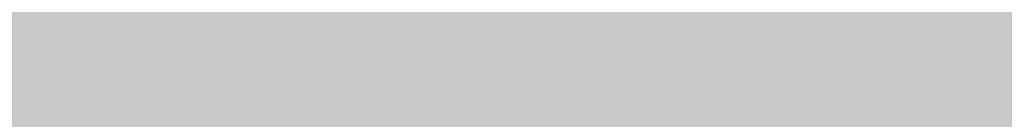
# Model space of a CAD drawing. Units: millimetres. Extents: x 0 to 2267, y 0 to 1823.
# Tile 104 of 256: x 1600.369 to 1605.705, y 1231.521 to 1232.061. Entities that reach past the tile are written whole.
import ezdxf

# ---------------------------------------------------------------- set-up
doc = ezdxf.new("R2010")
doc.units = ezdxf.units.MM
doc.header["$MEASUREMENT"] = 0
doc.layers.add('M-DIMS', color=2, linetype='Continuous', lineweight=25)
doc.layers.add('M-HATC', color=252, linetype='Continuous', lineweight=18)
doc.styles.get("Standard").update_dxf_attribs({"font": 'arial.ttf'})
doc.dimstyles.get("Standard").update_dxf_attribs({"dimtxt": 7, "dimasz": 4, "dimexe": 0.18, "dimexo": 0.0625, "dimgap": 0.09, "dimtad": 0, "dimdec": 0, "dimzin": 0, "dimdsep": 46, "dimtxsty": 'Standard', "dimcen": 0.09, "dimadec": 0, "dimazin": 0, "dimtfac": 1, "dimtdec": 0, "dimtofl": 0, "dimtmove": 0, "dimatfit": 3, "dimfxl": 1, "dimtolj": 1, "dimtzin": 0, "dimarcsym": 0})

# ---------------------------------------------------------------- blocks, each defined once
blk = doc.blocks.new('*D19')
at = {"layer": 'Defpoints', "color": 0, "transparency": 16777216}
for p in [(1605.3399, 1483.3044), (1445.5291, 1333.8851)]:
    blk.add_point(p, dxfattribs=at)
at = {"layer": 'M-DIMS', "color": 0, "lineweight": -2, "transparency": 16777216}
for p, q in [((1605.3399, 1483.2144), (1605.3399, 1483.3944)), ((1605.2499, 1483.3044), (1605.4299, 1483.3044)), ((1366.3244, 1259.8306), (1442.6072, 1331.1532))]:
    blk.add_line(p, q, dxfattribs=at)
at = {"layer": 'M-DIMS', "color": 0, "transparency": 16777216}
blk.add_solid([(1442.1519, 1331.6402), (1443.0625, 1330.6663), (1445.5291, 1333.8851)], dxfattribs=at)
at = {"layer": 'M-DIMS', "color": 0, "transparency": 16777216, "insert": (1349.6425, 1244.2335), "char_height": 7, "attachment_point": 5, "rotation": 43.0753}
blk.add_mtext('\\A1;2X R218.8', dxfattribs=at)

msp = doc.modelspace()

# ---------------------------------------------------------------- hatches: boundary and pattern name
at = {"layer": 'M-HATC'}
h = msp.add_hatch(color=256, dxfattribs=at)
h.dxf.hatch_style = 1
h.paths.add_polyline_path([(2055.771, 1603.062), (1381.0868, 1603.062), (1381.0868, 1598.062), (2055.771, 1598.062)])
h.paths.add_polyline_path([(2055.771, 1598.062), (1381.0868, 1598.062), (1381.0868, 1593.062), (2055.771, 1593.062)])
h.paths.add_polyline_path([(2051.3074, 1536.7609), (1385.5504, 1536.7609), (1385.5504, 1526.7609), (1387.5504, 1526.7609), (1388.5366, 1525.0528), (1385.3319, 1521.2335), (1385.3319, 1521.2226), (2050.2542, 1522.7491), (2048.3212, 1525.0528), (2049.3074, 1526.7609), (2051.3074, 1526.7609)])
edge = h.paths.add_edge_path()
edge.add_arc((1847.5345, 1379.1492), 135, 222.603061, 222.890851, ccw=False)
edge.add_line((1748.1663, 1287.7656), (1683.0921, 1287.7656))
edge.add_arc((1583.7239, 1379.1492), 135, 317.109149, 317.396939, ccw=False)
edge.add_arc((1678.9686, 1290.6707), 5, 222.8909, 317.1091, ccw=False)
edge.add_arc((1774.2133, 1379.1492), 135, 222.603061, 222.890851, ccw=False)
edge.add_line((1674.8451, 1287.7656), (1609.7709, 1287.7656))
edge.add_arc((1510.4027, 1379.1492), 135, 317.109149, 317.396939, ccw=False)
edge.add_arc((1605.6474, 1290.6707), 5, 222.8909, 317.1091, ccw=False)
edge.add_arc((1700.8921, 1379.1492), 135, 222.603061, 222.890851, ccw=False)
edge.add_line((1601.5239, 1287.7656), (1536.4497, 1287.7656))
edge.add_arc((1437.0815, 1379.1492), 135, 317.109149, 317.396939, ccw=False)
edge.add_arc((1532.3262, 1290.6707), 5, 222.8909, 317.1091, ccw=False)
edge.add_arc((1627.5709, 1379.1492), 135, 222.603061, 222.890851, ccw=False)
edge.add_line((1528.2027, 1287.7656), (1505.9289, 1287.7656))
edge.add_spline(control_points=[(1505.9289, 1287.7656), (1504.2622, 1287.7656), (1504.2622, 1282.7656), (1505.9289, 1282.7656)], knot_values=[0, 0, 0, 0, 5, 5, 5, 5], degree=3, periodic=0)
edge.add_line((1505.9289, 1282.7656), (1930.9289, 1282.7656))
edge.add_spline(control_points=[(1930.9289, 1282.7656), (1932.5956, 1282.7656), (1932.5956, 1287.7656), (1930.9289, 1287.7656)], knot_values=[0, 0, 0, 0, 5, 5, 5, 5], degree=3, periodic=0)
edge.add_line((1930.9289, 1287.7656), (1903.0557, 1287.7656))
edge.add_arc((1803.6875, 1379.1492), 135, 317.109149, 317.396939, ccw=False)
edge.add_arc((1898.9322, 1290.6707), 5, 222.8909, 317.1091, ccw=False)
edge.add_arc((1994.1769, 1379.1492), 135, 222.603061, 222.890851, ccw=False)
edge.add_line((1894.8087, 1287.7656), (1829.7345, 1287.7656))
edge.add_arc((1730.3663, 1379.1492), 135, 317.109149, 317.396939, ccw=False)
edge.add_arc((1825.611, 1290.6707), 5, 222.8909, 317.1091, ccw=False)
edge.add_arc((1920.8557, 1379.1492), 135, 222.603061, 222.890851, ccw=False)
edge.add_line((1821.4875, 1287.7656), (1756.4133, 1287.7656))
edge.add_arc((1657.0451, 1379.1492), 135, 317.109149, 317.396939, ccw=False)
edge.add_arc((1752.2898, 1290.6707), 5, 222.8909, 317.1091, ccw=False)
edge = h.paths.add_edge_path()
edge.add_spline(control_points=[(1843.4289, 1227.2475), (1845.0956, 1227.2475), (1845.0956, 1232.2475), (1843.4289, 1232.2475)], knot_values=[0, 0, 0, 0, 5, 5, 5, 5], degree=3, periodic=0)
edge.add_line((1843.4289, 1232.2475), (1593.4289, 1232.2475))
edge.add_spline(control_points=[(1593.4289, 1232.2475), (1591.7622, 1232.2475), (1591.7622, 1227.2475), (1593.4289, 1227.2475)], knot_values=[0, 0, 0, 0, 5, 5, 5, 5], degree=3, periodic=0)
edge.add_line((1593.4289, 1227.2475), (1843.4289, 1227.2475))
h.paths.add_polyline_path([(1905.9289, 1127.4171), (1530.9289, 1127.4171, 0.414214), (1520.9289, 1117.4171), (1530.9289, 1117.4171), (1915.9289, 1117.4171, 0.414214)])
edge = h.paths.add_edge_path()
edge.add_arc((1397.0858, 1498.4078), 12.7299, 90.78215, 190.87871, ccw=False)
edge.add_line((1396.912, 1511.1365), (1428.0097, 1511.3488))
edge.add_line((1428.0097, 1511.3488), (1433.0097, 1511.3488))
edge.add_line((1433.0097, 1511.3488), (1434.439, 1511.3488))
edge.add_arc((1419.474, 1498.0804), 20, 41.561, 74.08211)
edge.add_line((1424.9592, 1517.3135), (1399.9351, 1517.2561))
edge.add_spline(control_points=[(1399.9307, 1517.2561), (1399.884, 1517.2131), (1399.8328, 1517.1689), (1399.7774, 1517.1236)], knot_values=[11.567499, 11.567499, 11.567499, 11.567499, 11.814249, 11.814249, 11.814249, 11.814249], degree=3, periodic=0)
edge.add_spline(control_points=[(1399.6328, 1517.0099), (1399.5831, 1516.9721), (1399.5307, 1516.9338), (1399.4759, 1516.8947)], knot_values=[11.167718, 11.167718, 11.167718, 11.167718, 11.365188, 11.365188, 11.365188, 11.365188], degree=3, periodic=0)
edge.add_spline(control_points=[(1399.3398, 1516.8001), (1399.1514, 1516.6719), (1398.9384, 1516.5377), (1398.704, 1516.3994)], knot_values=[10.376405, 10.376405, 10.376405, 10.376405, 11.00994, 11.00994, 11.00994, 11.00994], degree=3, periodic=0)
edge.add_spline(control_points=[(1398.6572, 1516.3719), (1398.5789, 1516.326), (1398.4983, 1516.2797), (1398.4155, 1516.2331)], knot_values=[10.125175, 10.125175, 10.125175, 10.125175, 10.334406, 10.334406, 10.334406, 10.334406], degree=3, periodic=0)
edge.add_spline(control_points=[(1398.2642, 1516.1487), (1398.196, 1516.1111), (1398.1263, 1516.0732), (1398.0555, 1516.0351)], knot_values=[9.832246, 9.832246, 9.832246, 9.832246, 9.999658, 9.999658, 9.999658, 9.999658], degree=3, periodic=0)
edge.add_spline(control_points=[(1397.9987, 1516.0048), (1397.7312, 1515.8621), (1397.446, 1515.7171), (1397.1466, 1515.5714)], knot_values=[9.161808, 9.161808, 9.161808, 9.161808, 9.787769, 9.787769, 9.787769, 9.787769], degree=3, periodic=0)
edge.add_spline(control_points=[(1397.1466, 1515.5714), (1396.8418, 1515.423), (1396.5222, 1515.274), (1396.1914, 1515.1262)], knot_values=[8.524455, 8.524455, 8.524455, 8.524455, 9.161808, 9.161808, 9.161808, 9.161808], degree=3, periodic=0)
edge.add_spline(control_points=[(1396.0777, 1515.0756), (1395.9854, 1515.0348), (1395.8922, 1514.994), (1395.7983, 1514.9534)], knot_values=[8.275193, 8.275193, 8.275193, 8.275193, 8.451726, 8.451726, 8.451726, 8.451726], degree=3, periodic=0)
edge.add_spline(control_points=[(1395.6018, 1514.8691), (1395.4997, 1514.8257), (1395.3968, 1514.7824), (1395.2932, 1514.7394)], knot_values=[7.962917, 7.962917, 7.962917, 7.962917, 8.152764, 8.152764, 8.152764, 8.152764], degree=3, periodic=0)
edge.add_spline(control_points=[(1395.2116, 1514.7057), (1394.8278, 1514.5475), (1394.4345, 1514.3929), (1394.0364, 1514.2442)], knot_values=[7.21254, 7.21254, 7.21254, 7.21254, 7.913148, 7.913148, 7.913148, 7.913148], degree=3, periodic=0)
edge.add_spline(control_points=[(1394.0364, 1514.2442), (1393.7076, 1514.1214), (1393.3754, 1514.0027), (1393.0427, 1513.8895)], knot_values=[6.633733, 6.633733, 6.633733, 6.633733, 7.21254, 7.21254, 7.21254, 7.21254], degree=3, periodic=0)
edge.add_spline(control_points=[(1392.8214, 1513.815), (1392.7198, 1513.7812), (1392.6181, 1513.7479), (1392.5166, 1513.7152)], knot_values=[6.328796, 6.328796, 6.328796, 6.328796, 6.505493, 6.505493, 6.505493, 6.505493], degree=3, periodic=0)
edge.add_spline(control_points=[(1392.5166, 1513.7152), (1392.3187, 1513.6515), (1392.1212, 1513.59), (1391.9244, 1513.531)], knot_values=[5.984605, 5.984605, 5.984605, 5.984605, 6.328796, 6.328796, 6.328796, 6.328796], degree=3, periodic=0)
edge.add_spline(control_points=[(1391.7915, 1513.4915), (1391.3122, 1513.3501), (1390.8384, 1513.2239), (1390.3784, 1513.1171)], knot_values=[5.066697, 5.066697, 5.066697, 5.066697, 5.907055, 5.907055, 5.907055, 5.907055], degree=3, periodic=0)
edge.add_spline(control_points=[(1390.3784, 1513.1171), (1390.1797, 1513.071), (1389.9836, 1513.0284), (1389.7907, 1512.9899)], knot_values=[4.70367, 4.70367, 4.70367, 4.70367, 5.066695, 5.066695, 5.066695, 5.066695], degree=3, periodic=0)
edge.add_spline(control_points=[(1389.422, 1512.9204), (1389.2459, 1512.8892), (1389.0729, 1512.8617), (1388.9036, 1512.8381)], knot_values=[4.130571, 4.130571, 4.130571, 4.130571, 4.469816, 4.469816, 4.469816, 4.469816], degree=3, periodic=0)
edge.add_spline(control_points=[(1388.9036, 1512.8381), (1388.591, 1512.7946), (1388.2911, 1512.7644), (1388.0071, 1512.7494)], knot_values=[3.504031, 3.504031, 3.504031, 3.504031, 4.130571, 4.130571, 4.130571, 4.130571], degree=3, periodic=0)
edge.add_spline(control_points=[(1387.9356, 1512.7459), (1387.8538, 1512.7423), (1387.7733, 1512.74), (1387.6944, 1512.739)], knot_values=[3.268866, 3.268866, 3.268866, 3.268866, 3.451164, 3.451164, 3.451164, 3.451164], degree=3, periodic=0)
edge.add_spline(control_points=[(1387.3351, 1512.7443), (1387.2076, 1512.7499), (1387.0847, 1512.7597), (1386.967, 1512.7739)], knot_values=[2.670686, 2.670686, 2.670686, 2.670686, 2.984, 2.984, 2.984, 2.984], degree=3, periodic=0)
edge.add_spline(control_points=[(1386.8327, 1512.7922), (1386.8209, 1512.7941), (1386.8092, 1512.7959), (1386.7975, 1512.7979)], knot_values=[2.516981, 2.516981, 2.516981, 2.516981, 2.549528, 2.549528, 2.549528, 2.549528], degree=3, periodic=0)
edge.add_spline(control_points=[(1386.4526, 1512.8735), (1386.4257, 1512.881), (1386.3993, 1512.889), (1386.3733, 1512.8972)], knot_values=[2.095869, 2.095869, 2.095869, 2.095869, 2.17941, 2.17941, 2.17941, 2.17941], degree=3, periodic=0)
edge.add_spline(control_points=[(1386.0691, 1513.0189), (1386.0634, 1513.0217), (1386.0577, 1513.0246), (1386.052, 1513.0275)], knot_values=[1.72453, 1.72453, 1.72453, 1.72453, 1.745933, 1.745933, 1.745933, 1.745933], degree=3, periodic=0)
edge.add_arc((1399.474, 1498.0804), 20, 131.82432, 180)
edge.add_arc((1630.3336, 1505.5484), 250.9708, 181.705176, 236.427975)
edge.add_arc((1605.3399, 1483.3044), 218.7822, 238.660829, 243.34961)
edge.add_arc((1647.0911, 1510.3592), 262.8986, 183.129836, 237.853442, ccw=False)
h.paths.add_polyline_path([(1406.5369, 1391.9644, 0.149382), (1491.5506, 1296.4418, -0.129517)], flags=17)
edge = h.paths.add_edge_path()
edge.add_arc((2037.3838, 1498.0804), 20, 0, 48.26587)
edge.add_spline(control_points=[(2050.6973, 1513.0052), (2050.6512, 1512.9847), (2050.6034, 1512.9655), (2050.5539, 1512.9477)], knot_values=[1.835652, 1.835652, 1.835652, 1.835652, 2.000781, 2.000781, 2.000781, 2.000781], degree=3, periodic=0)
edge.add_spline(control_points=[(2050.4616, 1512.9166), (2050.479, 1512.9221), (2050.4963, 1512.9277), (2050.5133, 1512.9335)], knot_values=[2.045477, 2.045477, 2.045477, 2.045477, 2.101389, 2.101389, 2.101389, 2.101389], degree=3, periodic=0)
edge.add_spline(control_points=[(2050.129, 1512.8342), (2050.1984, 1512.8473), (2050.2657, 1512.8623), (2050.3308, 1512.8792)], knot_values=[2.237629, 2.237629, 2.237629, 2.237629, 2.435841, 2.435841, 2.435841, 2.435841], degree=3, periodic=0)
edge.add_spline(control_points=[(2050.0946, 1512.8278), (2050.1061, 1512.8299), (2050.1176, 1512.832), (2050.129, 1512.8342)], knot_values=[2.435841, 2.435841, 2.435841, 2.435841, 2.468321, 2.468321, 2.468321, 2.468321], degree=3, periodic=0)
edge.add_spline(control_points=[(2049.7843, 1512.7851), (2049.8552, 1512.7922), (2049.9243, 1512.8008), (2049.9917, 1512.8109)], knot_values=[2.563852, 2.563852, 2.563852, 2.563852, 2.748541, 2.748541, 2.748541, 2.748541], degree=3, periodic=0)
edge.add_spline(control_points=[(2049.4052, 1512.7617), (2049.5364, 1512.7653), (2049.6629, 1512.773), (2049.7843, 1512.7851)], knot_values=[2.748541, 2.748541, 2.748541, 2.748541, 3.064882, 3.064882, 3.064882, 3.064882], degree=3, periodic=0)
edge.add_spline(control_points=[(2049.1698, 1512.7597), (2049.2336, 1512.7591), (2049.2965, 1512.7594), (2049.3584, 1512.7606)], knot_values=[3.102309, 3.102309, 3.102309, 3.102309, 3.2503, 3.2503, 3.2503, 3.2503], degree=3, periodic=0)
edge.add_spline(control_points=[(2048.8573, 1512.7691), (2048.9638, 1512.7638), (2049.068, 1512.7606), (2049.1698, 1512.7597)], knot_values=[3.2503, 3.2503, 3.2503, 3.2503, 3.486069, 3.486069, 3.486069, 3.486069], degree=3, periodic=0)
edge.add_spline(control_points=[(2048.6924, 1512.7789), (2048.3729, 1512.8009), (2048.0345, 1512.8411), (2047.6817, 1512.897)], knot_values=[3.606429, 3.606429, 3.606429, 3.606429, 4.2989, 4.2989, 4.2989, 4.2989], degree=3, periodic=0)
edge.add_spline(control_points=[(2047.6817, 1512.897), (2047.5458, 1512.9185), (2047.4077, 1512.9424), (2047.2678, 1512.9685)], knot_values=[4.2989, 4.2989, 4.2989, 4.2989, 4.565769, 4.565769, 4.565769, 4.565769], degree=3, periodic=0)
edge.add_spline(control_points=[(2047.2678, 1512.9685), (2047.1449, 1512.9914), (2047.0207, 1513.016), (2046.8951, 1513.0422)], knot_values=[4.565769, 4.565769, 4.565769, 4.565769, 4.799971, 4.799971, 4.799971, 4.799971], degree=3, periodic=0)
edge.add_spline(control_points=[(2046.8951, 1513.0422), (2046.5286, 1513.1188), (2046.1513, 1513.209), (2045.7676, 1513.3107)], knot_values=[4.799971, 4.799971, 4.799971, 4.799971, 5.483718, 5.483718, 5.483718, 5.483718], degree=3, periodic=0)
edge.add_spline(control_points=[(2045.7676, 1513.3107), (2045.3724, 1513.4154), (2044.9704, 1513.5322), (2044.5662, 1513.6588)], knot_values=[5.483718, 5.483718, 5.483718, 5.483718, 6.187866, 6.187866, 6.187866, 6.187866], degree=3, periodic=0)
edge.add_spline(control_points=[(2044.5662, 1513.6588), (2044.4149, 1513.7061), (2044.2633, 1513.7549), (2044.1116, 1513.8048)], knot_values=[6.187866, 6.187866, 6.187866, 6.187866, 6.451551, 6.451551, 6.451551, 6.451551], degree=3, periodic=0)
edge.add_spline(control_points=[(2044.1116, 1513.8048), (2043.9967, 1513.8427), (2043.8817, 1513.8813), (2043.7668, 1513.9205)], knot_values=[6.451551, 6.451551, 6.451551, 6.451551, 6.651434, 6.651434, 6.651434, 6.651434], degree=3, periodic=0)
edge.add_spline(control_points=[(2043.7668, 1513.9205), (2043.3716, 1514.0554), (2042.9774, 1514.1979), (2042.5886, 1514.3458)], knot_values=[6.651434, 6.651434, 6.651434, 6.651434, 7.338879, 7.338879, 7.338879, 7.338879], degree=3, periodic=0)
edge.add_spline(control_points=[(2042.5886, 1514.3458), (2042.1643, 1514.5071), (2041.7465, 1514.6749), (2041.3409, 1514.846)], knot_values=[7.338879, 7.338879, 7.338879, 7.338879, 8.089209, 8.089209, 8.089209, 8.089209], degree=3, periodic=0)
edge.add_spline(control_points=[(2041.3409, 1514.846), (2041.1028, 1514.9465), (2040.869, 1515.0481), (2040.6405, 1515.1502)], knot_values=[8.089209, 8.089209, 8.089209, 8.089209, 8.529587, 8.529587, 8.529587, 8.529587], degree=3, periodic=0)
edge.add_spline(control_points=[(2040.51, 1515.2089), (2040.0824, 1515.4022), (2039.6747, 1515.5971), (2039.295, 1515.7894)], knot_values=[8.613818, 8.613818, 8.613818, 8.613818, 9.44571, 9.44571, 9.44571, 9.44571], degree=3, periodic=0)
edge.add_spline(control_points=[(2039.295, 1515.7894), (2039.0618, 1515.9075), (2038.8391, 1516.0246), (2038.6288, 1516.1398)], knot_values=[9.44571, 9.44571, 9.44571, 9.44571, 9.956404, 9.956404, 9.956404, 9.956404], degree=3, periodic=0)
edge.add_spline(control_points=[(2038.6288, 1516.1398), (2038.5187, 1516.2001), (2038.4121, 1516.2598), (2038.309, 1516.3189)], knot_values=[9.956404, 9.956404, 9.956404, 9.956404, 10.223542, 10.223542, 10.223542, 10.223542], degree=3, periodic=0)
edge.add_spline(control_points=[(2038.309, 1516.3189), (2038.2138, 1516.3735), (2038.1216, 1516.4276), (2038.0328, 1516.481)], knot_values=[10.223542, 10.223542, 10.223542, 10.223542, 10.47051, 10.47051, 10.47051, 10.47051], degree=3, periodic=0)
edge.add_spline(control_points=[(2038.0328, 1516.481), (2037.7855, 1516.6296), (2037.5639, 1516.773), (2037.3722, 1516.909)], knot_values=[10.47051, 10.47051, 10.47051, 10.47051, 11.15767, 11.15767, 11.15767, 11.15767], degree=3, periodic=0)
edge.add_spline(control_points=[(2037.3722, 1516.909), (2037.2789, 1516.9752), (2037.1927, 1517.0396), (2037.1142, 1517.102)], knot_values=[11.15767, 11.15767, 11.15767, 11.15767, 11.49227, 11.49227, 11.49227, 11.49227], degree=3, periodic=0)
edge.add_spline(control_points=[(2036.8564, 1517.3259), (2036.9148, 1517.2692), (2036.9814, 1517.2103), (2037.0557, 1517.1492)], knot_values=[11.577341, 11.577341, 11.577341, 11.577341, 11.91035, 11.91035, 11.91035, 11.91035], degree=3, periodic=0)
edge.add_spline(control_points=[(2036.8074, 1517.3748), (2036.823, 1517.3587), (2036.8393, 1517.3424), (2036.8564, 1517.3259)], knot_values=[11.91035, 11.91035, 11.91035, 11.91035, 12.007402, 12.007402, 12.007402, 12.007402], degree=3, periodic=0)
edge.add_spline(control_points=[(2036.7017, 1517.494), (2036.7104, 1517.483), (2036.7196, 1517.4719), (2036.7291, 1517.4606)], knot_values=[12.184155, 12.184155, 12.184155, 12.184155, 12.255409, 12.255409, 12.255409, 12.255409], degree=3, periodic=0)
edge.add_spline(control_points=[(2036.6159, 1517.6205), (2036.62, 1517.613), (2036.6243, 1517.6055), (2036.6289, 1517.5979)], knot_values=[12.487913, 12.487913, 12.487913, 12.487913, 12.541035, 12.541035, 12.541035, 12.541035], degree=3, periodic=0)
edge.add_spline(control_points=[(2036.5635, 1517.786), (2036.5637, 1517.7794), (2036.5642, 1517.7726), (2036.565, 1517.7658)], knot_values=[12.911761, 12.911761, 12.911761, 12.911761, 12.968286, 12.968286, 12.968286, 12.968286], degree=3, periodic=0)
edge.add_spline(control_points=[(2036.6166, 1517.9304), (2036.6125, 1517.9259), (2036.6086, 1517.9212), (2036.6049, 1517.9165)], knot_values=[13.382527, 13.382527, 13.382527, 13.382527, 13.433791, 13.433791, 13.433791, 13.433791], degree=3, periodic=0)
edge.add_spline(control_points=[(2036.749, 1518.017), (2036.7361, 1518.0116), (2036.7239, 1518.006), (2036.7124, 1518.0002)], knot_values=[13.726299, 13.726299, 13.726299, 13.726299, 13.809928, 13.809928, 13.809928, 13.809928], degree=3, periodic=0)
edge.add_spline(control_points=[(2036.8604, 1518.0528), (2036.8386, 1518.0474), (2036.8181, 1518.0416), (2036.7988, 1518.0353)], knot_values=[13.910887, 13.910887, 13.910887, 13.910887, 14.02153, 14.02153, 14.02153, 14.02153], degree=3, periodic=0)
edge.add_line((2036.9639, 1518.0804), (2032.3838, 1518.0804))
edge.add_line((2032.3838, 1518.0804), (2027.3838, 1518.0804))
edge.add_line((2027.3838, 1518.0804), (2022.3838, 1518.0804))
edge.add_line((2022.3838, 1518.0804), (2017.3838, 1518.0804))
edge.add_arc((2017.3838, 1498.0804), 20, 90, 138.439)
edge.add_line((2002.4188, 1511.3488), (2003.8481, 1511.3488))
edge.add_line((2003.8481, 1511.3488), (2008.8481, 1511.3488))
edge.add_line((2008.8481, 1511.3488), (2039.772, 1511.1377))
edge.add_arc((2039.772, 1498.4078), 12.7299, -10.87871, 90, ccw=False)
edge.add_arc((1789.7668, 1510.3592), 262.8986, 302.146558, 356.870164, ccw=False)
edge.add_arc((1831.5179, 1483.3044), 218.7822, 296.65039, 301.339171)
edge.add_arc((1806.5242, 1505.5484), 250.9708, 303.572025, 358.294824)
h.paths.add_polyline_path([(2030.321, 1391.9644, -0.129517), (1945.3072, 1296.4418, 0.149382)], flags=17)
edge = h.paths.add_edge_path()
edge.add_spline(control_points=[(2037.2464, 1518.0821), (2037.2898, 1518.081), (2037.3355, 1518.0804), (2037.3838, 1518.0804)], knot_values=[0.000012, 0.000012, 0.000012, 0.000012, 0.144754, 0.144754, 0.144754, 0.144754], degree=3, periodic=0)
edge.add_line((2037.3357, 1518.0804), (2037.0096, 1518.0804))
edge.add_spline(control_points=[(2037.0096, 1518.0804), (2036.9822, 1518.0768), (2036.956, 1518.0727), (2036.9312, 1518.0681)], knot_values=[14.13465, 14.13465, 14.13465, 14.13465, 14.247197, 14.247197, 14.247197, 14.247197], degree=3, periodic=0)
edge.add_spline(control_points=[(2036.9312, 1518.0681), (2036.9276, 1518.0674), (2036.9241, 1518.0667), (2036.9205, 1518.0661)], knot_values=[14.118315, 14.118315, 14.118315, 14.118315, 14.13465, 14.13465, 14.13465, 14.13465], degree=3, periodic=0)
edge.add_spline(control_points=[(2036.9205, 1518.0661), (2036.9118, 1518.0644), (2036.9032, 1518.0626), (2036.8948, 1518.0608)], knot_values=[14.078086, 14.078086, 14.078086, 14.078086, 14.118315, 14.118315, 14.118315, 14.118315], degree=3, periodic=0)
edge.add_spline(control_points=[(2036.8948, 1518.0608), (2036.883, 1518.0583), (2036.8716, 1518.0556), (2036.8604, 1518.0528)], knot_values=[14.02153, 14.02153, 14.02153, 14.02153, 14.078086, 14.078086, 14.078086, 14.078086], degree=3, periodic=0)
edge.add_spline(control_points=[(2036.8604, 1518.0528), (2036.8386, 1518.0474), (2036.8181, 1518.0416), (2036.7988, 1518.0353)], knot_values=[13.910887, 13.910887, 13.910887, 13.910887, 14.02153, 14.02153, 14.02153, 14.02153], degree=3, periodic=0)
edge.add_spline(control_points=[(2036.7988, 1518.0353), (2036.7981, 1518.035), (2036.7974, 1518.0348), (2036.7967, 1518.0346)], knot_values=[13.906906, 13.906906, 13.906906, 13.906906, 13.910887, 13.910887, 13.910887, 13.910887], degree=3, periodic=0)
edge.add_spline(control_points=[(2036.7967, 1518.0346), (2036.7882, 1518.0318), (2036.7799, 1518.0289), (2036.7719, 1518.0259)], knot_values=[13.857826, 13.857826, 13.857826, 13.857826, 13.906906, 13.906906, 13.906906, 13.906906], degree=3, periodic=0)
edge.add_spline(control_points=[(2036.7719, 1518.0259), (2036.764, 1518.023), (2036.7564, 1518.02), (2036.749, 1518.017)], knot_values=[13.809928, 13.809928, 13.809928, 13.809928, 13.857826, 13.857826, 13.857826, 13.857826], degree=3, periodic=0)
edge.add_spline(control_points=[(2036.749, 1518.017), (2036.7361, 1518.0116), (2036.7239, 1518.006), (2036.7124, 1518.0002)], knot_values=[13.726299, 13.726299, 13.726299, 13.726299, 13.809928, 13.809928, 13.809928, 13.809928], degree=3, periodic=0)
edge.add_spline(control_points=[(2036.7124, 1518.0002), (2036.7121, 1518), (2036.7118, 1517.9999), (2036.7115, 1517.9997)], knot_values=[13.723993, 13.723993, 13.723993, 13.723993, 13.726299, 13.726299, 13.726299, 13.726299], degree=3, periodic=0)
edge.add_spline(control_points=[(2036.7115, 1517.9997), (2036.7063, 1517.9971), (2036.7013, 1517.9944), (2036.6965, 1517.9917)], knot_values=[13.686536, 13.686536, 13.686536, 13.686536, 13.723993, 13.723993, 13.723993, 13.723993], degree=3, periodic=0)
edge.add_spline(control_points=[(2036.6965, 1517.9917), (2036.6919, 1517.9891), (2036.6874, 1517.9865), (2036.6831, 1517.9839)], knot_values=[13.651251, 13.651251, 13.651251, 13.651251, 13.686536, 13.686536, 13.686536, 13.686536], degree=3, periodic=0)
edge.add_spline(control_points=[(2036.6831, 1517.9839), (2036.6764, 1517.9798), (2036.67, 1517.9757), (2036.6639, 1517.9714)], knot_values=[13.596804, 13.596804, 13.596804, 13.596804, 13.651251, 13.651251, 13.651251, 13.651251], degree=3, periodic=0)
edge.add_spline(control_points=[(2036.6639, 1517.9714), (2036.6636, 1517.9712), (2036.6633, 1517.9709), (2036.6629, 1517.9707)], knot_values=[13.593956, 13.593956, 13.593956, 13.593956, 13.596804, 13.596804, 13.596804, 13.596804], degree=3, periodic=0)
edge.add_spline(control_points=[(2036.6629, 1517.9707), (2036.6603, 1517.9689), (2036.6577, 1517.967), (2036.6552, 1517.9651)], knot_values=[13.570322, 13.570322, 13.570322, 13.570322, 13.593956, 13.593956, 13.593956, 13.593956], degree=3, periodic=0)
edge.add_spline(control_points=[(2036.6552, 1517.9651), (2036.6525, 1517.9631), (2036.6499, 1517.9611), (2036.6474, 1517.9591)], knot_values=[13.545477, 13.545477, 13.545477, 13.545477, 13.570322, 13.570322, 13.570322, 13.570322], degree=3, periodic=0)
edge.add_spline(control_points=[(2036.6474, 1517.9591), (2036.6472, 1517.9589), (2036.6471, 1517.9588), (2036.6469, 1517.9587)], knot_values=[13.543931, 13.543931, 13.543931, 13.543931, 13.545477, 13.545477, 13.545477, 13.545477], degree=3, periodic=0)
edge.add_spline(control_points=[(2036.6469, 1517.9587), (2036.6412, 1517.9541), (2036.6358, 1517.9494), (2036.6307, 1517.9447)], knot_values=[13.488237, 13.488237, 13.488237, 13.488237, 13.543931, 13.543931, 13.543931, 13.543931], degree=3, periodic=0)
edge.add_spline(control_points=[(2036.6307, 1517.9447), (2036.6282, 1517.9423), (2036.6257, 1517.9399), (2036.6233, 1517.9374)], knot_values=[13.460307, 13.460307, 13.460307, 13.460307, 13.488237, 13.488237, 13.488237, 13.488237], degree=3, periodic=0)
edge.add_spline(control_points=[(2036.6233, 1517.9374), (2036.6215, 1517.9356), (2036.6198, 1517.9338), (2036.6181, 1517.932)], knot_values=[13.439712, 13.439712, 13.439712, 13.439712, 13.460307, 13.460307, 13.460307, 13.460307], degree=3, periodic=0)
edge.add_spline(control_points=[(2036.6181, 1517.932), (2036.6176, 1517.9315), (2036.6171, 1517.9309), (2036.6166, 1517.9304)], knot_values=[13.433791, 13.433791, 13.433791, 13.433791, 13.439712, 13.439712, 13.439712, 13.439712], degree=3, periodic=0)
edge.add_spline(control_points=[(2036.6166, 1517.9304), (2036.6125, 1517.9259), (2036.6086, 1517.9212), (2036.6049, 1517.9165)], knot_values=[13.382527, 13.382527, 13.382527, 13.382527, 13.433791, 13.433791, 13.433791, 13.433791], degree=3, periodic=0)
edge.add_spline(control_points=[(2036.6049, 1517.9165), (2036.6026, 1517.9135), (2036.6004, 1517.9104), (2036.5982, 1517.9074)], knot_values=[13.350017, 13.350017, 13.350017, 13.350017, 13.382527, 13.382527, 13.382527, 13.382527], degree=3, periodic=0)
edge.add_spline(control_points=[(2036.5982, 1517.9074), (2036.5972, 1517.9059), (2036.5962, 1517.9043), (2036.5952, 1517.9028)], knot_values=[13.333922, 13.333922, 13.333922, 13.333922, 13.350017, 13.350017, 13.350017, 13.350017], degree=3, periodic=0)
edge.add_spline(control_points=[(2036.5952, 1517.9028), (2036.5945, 1517.9018), (2036.5939, 1517.9009), (2036.5933, 1517.8999)], knot_values=[13.323828, 13.323828, 13.323828, 13.323828, 13.333922, 13.333922, 13.333922, 13.333922], degree=3, periodic=0)
edge.add_spline(control_points=[(2036.5933, 1517.8999), (2036.5905, 1517.8955), (2036.5879, 1517.8909), (2036.5855, 1517.8864)], knot_values=[13.277545, 13.277545, 13.277545, 13.277545, 13.323828, 13.323828, 13.323828, 13.323828], degree=3, periodic=0)
edge.add_spline(control_points=[(2036.5855, 1517.8864), (2036.5836, 1517.8827), (2036.5817, 1517.8789), (2036.5801, 1517.8751)], knot_values=[13.240119, 13.240119, 13.240119, 13.240119, 13.277545, 13.277545, 13.277545, 13.277545], degree=3, periodic=0)
edge.add_spline(control_points=[(2036.5801, 1517.8751), (2036.5795, 1517.8739), (2036.579, 1517.8727), (2036.5785, 1517.8715)], knot_values=[13.228211, 13.228211, 13.228211, 13.228211, 13.240119, 13.240119, 13.240119, 13.240119], degree=3, periodic=0)
edge.add_spline(control_points=[(2036.5785, 1517.8715), (2036.578, 1517.8702), (2036.5774, 1517.869), (2036.5769, 1517.8677)], knot_values=[13.215717, 13.215717, 13.215717, 13.215717, 13.228211, 13.228211, 13.228211, 13.228211], degree=3, periodic=0)
edge.add_spline(control_points=[(2036.5769, 1517.8677), (2036.5755, 1517.864), (2036.5741, 1517.8603), (2036.5729, 1517.8565)], knot_values=[13.179847, 13.179847, 13.179847, 13.179847, 13.215717, 13.215717, 13.215717, 13.215717], degree=3, periodic=0)
edge.add_spline(control_points=[(2036.5729, 1517.8565), (2036.5713, 1517.8515), (2036.5699, 1517.8464), (2036.5687, 1517.8413)], knot_values=[13.132017, 13.132017, 13.132017, 13.132017, 13.179847, 13.179847, 13.179847, 13.179847], degree=3, periodic=0)
edge.add_spline(control_points=[(2036.5687, 1517.8413), (2036.5684, 1517.8402), (2036.5682, 1517.8392), (2036.568, 1517.8382)], knot_values=[13.122482, 13.122482, 13.122482, 13.122482, 13.132017, 13.132017, 13.132017, 13.132017], degree=3, periodic=0)
edge.add_spline(control_points=[(2036.568, 1517.8382), (2036.5676, 1517.8363), (2036.5672, 1517.8345), (2036.5669, 1517.8327)], knot_values=[13.105592, 13.105592, 13.105592, 13.105592, 13.122482, 13.122482, 13.122482, 13.122482], degree=3, periodic=0)
edge.add_spline(control_points=[(2036.5669, 1517.8327), (2036.5662, 1517.8292), (2036.5657, 1517.8257), (2036.5652, 1517.8222)], knot_values=[13.074063, 13.074063, 13.074063, 13.074063, 13.105592, 13.105592, 13.105592, 13.105592], degree=3, periodic=0)
edge.add_spline(control_points=[(2036.5652, 1517.8222), (2036.5652, 1517.8222), (2036.5652, 1517.8222), (2036.5652, 1517.8222)], knot_values=[13.074043, 13.074043, 13.074043, 13.074043, 13.074063, 13.074063, 13.074063, 13.074063], degree=3, periodic=0)
edge.add_spline(control_points=[(2036.5652, 1517.8222), (2036.5644, 1517.8164), (2036.5639, 1517.8106), (2036.5636, 1517.8046)], knot_values=[13.021884, 13.021884, 13.021884, 13.021884, 13.074043, 13.074043, 13.074043, 13.074043], degree=3, periodic=0)
edge.add_spline(control_points=[(2036.5636, 1517.8046), (2036.5636, 1517.804), (2036.5636, 1517.8034), (2036.5635, 1517.8028)], knot_values=[13.01674, 13.01674, 13.01674, 13.01674, 13.021884, 13.021884, 13.021884, 13.021884], degree=3, periodic=0)
edge.add_spline(control_points=[(2036.5635, 1517.8028), (2036.5634, 1517.8005), (2036.5634, 1517.7982), (2036.5634, 1517.7958)], knot_values=[12.996438, 12.996438, 12.996438, 12.996438, 13.01674, 13.01674, 13.01674, 13.01674], degree=3, periodic=0)
edge.add_spline(control_points=[(2036.5634, 1517.7958), (2036.5633, 1517.7926), (2036.5634, 1517.7893), (2036.5635, 1517.786)], knot_values=[12.968286, 12.968286, 12.968286, 12.968286, 12.996438, 12.996438, 12.996438, 12.996438], degree=3, periodic=0)
edge.add_spline(control_points=[(2036.5635, 1517.786), (2036.5637, 1517.7794), (2036.5642, 1517.7726), (2036.565, 1517.7658)], knot_values=[12.911761, 12.911761, 12.911761, 12.911761, 12.968286, 12.968286, 12.968286, 12.968286], degree=3, periodic=0)
edge.add_spline(control_points=[(2036.565, 1517.7658), (2036.565, 1517.7657), (2036.565, 1517.7656), (2036.565, 1517.7656)], knot_values=[12.911017, 12.911017, 12.911017, 12.911017, 12.911761, 12.911761, 12.911761, 12.911761], degree=3, periodic=0)
edge.add_spline(control_points=[(2036.565, 1517.7656), (2036.5654, 1517.7625), (2036.5658, 1517.7593), (2036.5663, 1517.7562)], knot_values=[12.88528, 12.88528, 12.88528, 12.88528, 12.911017, 12.911017, 12.911017, 12.911017], degree=3, periodic=0)
edge.add_spline(control_points=[(2036.5663, 1517.7562), (2036.5667, 1517.7534), (2036.5672, 1517.7506), (2036.5677, 1517.7478)], knot_values=[12.862519, 12.862519, 12.862519, 12.862519, 12.88528, 12.88528, 12.88528, 12.88528], degree=3, periodic=0)
edge.add_spline(control_points=[(2036.5677, 1517.7478), (2036.5678, 1517.7474), (2036.5679, 1517.7469), (2036.568, 1517.7465)], knot_values=[12.858885, 12.858885, 12.858885, 12.858885, 12.862519, 12.862519, 12.862519, 12.862519], degree=3, periodic=0)
edge.add_spline(control_points=[(2036.568, 1517.7465), (2036.5692, 1517.7399), (2036.5707, 1517.7332), (2036.5724, 1517.7264)], knot_values=[12.8053, 12.8053, 12.8053, 12.8053, 12.858885, 12.858885, 12.858885, 12.858885], degree=3, periodic=0)
edge.add_spline(control_points=[(2036.5724, 1517.7264), (2036.5734, 1517.7226), (2036.5745, 1517.7187), (2036.5756, 1517.7149)], knot_values=[12.775176, 12.775176, 12.775176, 12.775176, 12.8053, 12.8053, 12.8053, 12.8053], degree=3, periodic=0)
edge.add_spline(control_points=[(2036.5756, 1517.7149), (2036.5763, 1517.7125), (2036.577, 1517.7102), (2036.5778, 1517.7078)], knot_values=[12.756759, 12.756759, 12.756759, 12.756759, 12.775176, 12.775176, 12.775176, 12.775176], degree=3, periodic=0)
edge.add_spline(control_points=[(2036.5778, 1517.7078), (2036.5781, 1517.7067), (2036.5784, 1517.7057), (2036.5787, 1517.7047)], knot_values=[12.748742, 12.748742, 12.748742, 12.748742, 12.756759, 12.756759, 12.756759, 12.756759], degree=3, periodic=0)
edge.add_spline(control_points=[(2036.5787, 1517.7047), (2036.5808, 1517.6983), (2036.5831, 1517.6919), (2036.5856, 1517.6854)], knot_values=[12.69959, 12.69959, 12.69959, 12.69959, 12.748742, 12.748742, 12.748742, 12.748742], degree=3, periodic=0)
edge.add_spline(control_points=[(2036.5856, 1517.6854), (2036.5876, 1517.68), (2036.5898, 1517.6746), (2036.5921, 1517.6692)], knot_values=[12.659038, 12.659038, 12.659038, 12.659038, 12.69959, 12.69959, 12.69959, 12.69959], degree=3, periodic=0)
edge.add_spline(control_points=[(2036.5921, 1517.6692), (2036.594, 1517.6648), (2036.5959, 1517.6605), (2036.5979, 1517.6561)], knot_values=[12.626806, 12.626806, 12.626806, 12.626806, 12.659038, 12.659038, 12.659038, 12.659038], degree=3, periodic=0)
edge.add_spline(control_points=[(2036.5979, 1517.6561), (2036.5984, 1517.6551), (2036.5989, 1517.6541), (2036.5993, 1517.6531)], knot_values=[12.619394, 12.619394, 12.619394, 12.619394, 12.626806, 12.626806, 12.626806, 12.626806], degree=3, periodic=0)
edge.add_spline(control_points=[(2036.5993, 1517.6531), (2036.6043, 1517.6424), (2036.6099, 1517.6315), (2036.6159, 1517.6205)], knot_values=[12.541039, 12.541039, 12.541039, 12.541039, 12.619394, 12.619394, 12.619394, 12.619394], degree=3, periodic=0)
edge.add_spline(control_points=[(2036.6159, 1517.6205), (2036.6159, 1517.6205), (2036.6159, 1517.6205), (2036.6159, 1517.6205)], knot_values=[12.541035, 12.541035, 12.541035, 12.541035, 12.541039, 12.541039, 12.541039, 12.541039], degree=3, periodic=0)
edge.add_spline(control_points=[(2036.6159, 1517.6205), (2036.62, 1517.613), (2036.6243, 1517.6055), (2036.6289, 1517.5979)], knot_values=[12.487913, 12.487913, 12.487913, 12.487913, 12.541035, 12.541035, 12.541035, 12.541035], degree=3, periodic=0)
edge.add_spline(control_points=[(2036.6289, 1517.5979), (2036.6326, 1517.5916), (2036.6365, 1517.5853), (2036.6406, 1517.5789)], knot_values=[12.443982, 12.443982, 12.443982, 12.443982, 12.487913, 12.487913, 12.487913, 12.487913], degree=3, periodic=0)
edge.add_spline(control_points=[(2036.6406, 1517.5789), (2036.6414, 1517.5776), (2036.6423, 1517.5763), (2036.6431, 1517.5749)], knot_values=[12.434996, 12.434996, 12.434996, 12.434996, 12.443982, 12.443982, 12.443982, 12.443982], degree=3, periodic=0)
edge.add_spline(control_points=[(2036.6431, 1517.5749), (2036.6531, 1517.5596), (2036.6639, 1517.5439), (2036.6756, 1517.528)], knot_values=[12.329647, 12.329647, 12.329647, 12.329647, 12.434996, 12.434996, 12.434996, 12.434996], degree=3, periodic=0)
edge.add_spline(control_points=[(2036.6756, 1517.528), (2036.6839, 1517.5168), (2036.6925, 1517.5055), (2036.7017, 1517.494)], knot_values=[12.255409, 12.255409, 12.255409, 12.255409, 12.329647, 12.329647, 12.329647, 12.329647], degree=3, periodic=0)
edge.add_spline(control_points=[(2036.7017, 1517.494), (2036.7104, 1517.483), (2036.7196, 1517.4719), (2036.7291, 1517.4606)], knot_values=[12.184155, 12.184155, 12.184155, 12.184155, 12.255409, 12.255409, 12.255409, 12.255409], degree=3, periodic=0)
edge.add_spline(control_points=[(2036.7291, 1517.4606), (2036.7436, 1517.4435), (2036.759, 1517.4262), (2036.7753, 1517.4085)], knot_values=[12.075961, 12.075961, 12.075961, 12.075961, 12.184155, 12.184155, 12.184155, 12.184155], degree=3, periodic=0)
edge.add_spline(control_points=[(2036.7753, 1517.4085), (2036.7763, 1517.4075), (2036.7773, 1517.4064), (2036.7783, 1517.4054)], knot_values=[12.069502, 12.069502, 12.069502, 12.069502, 12.075961, 12.075961, 12.075961, 12.075961], degree=3, periodic=0)
edge.add_spline(control_points=[(2036.7783, 1517.4054), (2036.7877, 1517.3953), (2036.7974, 1517.385), (2036.8074, 1517.3748)], knot_values=[12.007402, 12.007402, 12.007402, 12.007402, 12.069502, 12.069502, 12.069502, 12.069502], degree=3, periodic=0)
edge.add_spline(control_points=[(2036.8074, 1517.3748), (2036.823, 1517.3587), (2036.8393, 1517.3424), (2036.8564, 1517.3259)], knot_values=[11.91035, 11.91035, 11.91035, 11.91035, 12.007402, 12.007402, 12.007402, 12.007402], degree=3, periodic=0)
edge.add_spline(control_points=[(2036.8564, 1517.3259), (2036.9148, 1517.2692), (2036.9814, 1517.2103), (2037.0557, 1517.1492)], knot_values=[11.577341, 11.577341, 11.577341, 11.577341, 11.91035, 11.91035, 11.91035, 11.91035], degree=3, periodic=0)
edge.add_spline(control_points=[(2037.0557, 1517.1492), (2037.0747, 1517.1336), (2037.0942, 1517.1179), (2037.1142, 1517.102)], knot_values=[11.49227, 11.49227, 11.49227, 11.49227, 11.577341, 11.577341, 11.577341, 11.577341], degree=3, periodic=0)
edge.add_spline(control_points=[(2037.1142, 1517.102), (2037.1927, 1517.0396), (2037.2789, 1516.9752), (2037.3722, 1516.909)], knot_values=[11.15767, 11.15767, 11.15767, 11.15767, 11.49227, 11.49227, 11.49227, 11.49227], degree=3, periodic=0)
edge.add_spline(control_points=[(2037.3722, 1516.909), (2037.5639, 1516.773), (2037.7855, 1516.6296), (2038.0328, 1516.481)], knot_values=[10.47051, 10.47051, 10.47051, 10.47051, 11.15767, 11.15767, 11.15767, 11.15767], degree=3, periodic=0)
edge.add_spline(control_points=[(2038.0328, 1516.481), (2038.1216, 1516.4276), (2038.2138, 1516.3735), (2038.309, 1516.3189)], knot_values=[10.223542, 10.223542, 10.223542, 10.223542, 10.47051, 10.47051, 10.47051, 10.47051], degree=3, periodic=0)
edge.add_spline(control_points=[(2038.309, 1516.3189), (2038.4121, 1516.2598), (2038.5187, 1516.2001), (2038.6288, 1516.1398)], knot_values=[9.956404, 9.956404, 9.956404, 9.956404, 10.223542, 10.223542, 10.223542, 10.223542], degree=3, periodic=0)
edge.add_spline(control_points=[(2038.6288, 1516.1398), (2038.8391, 1516.0246), (2039.0618, 1515.9075), (2039.295, 1515.7894)], knot_values=[9.44571, 9.44571, 9.44571, 9.44571, 9.956404, 9.956404, 9.956404, 9.956404], degree=3, periodic=0)
edge.add_spline(control_points=[(2039.295, 1515.7894), (2039.6747, 1515.5971), (2040.0824, 1515.4022), (2040.51, 1515.2089)], knot_values=[8.613818, 8.613818, 8.613818, 8.613818, 9.44571, 9.44571, 9.44571, 9.44571], degree=3, periodic=0)
edge.add_spline(control_points=[(2040.51, 1515.2089), (2040.5533, 1515.1893), (2040.5968, 1515.1697), (2040.6405, 1515.1502)], knot_values=[8.529587, 8.529587, 8.529587, 8.529587, 8.613818, 8.613818, 8.613818, 8.613818], degree=3, periodic=0)
edge.add_spline(control_points=[(2040.6405, 1515.1502), (2040.869, 1515.0481), (2041.1028, 1514.9465), (2041.3409, 1514.846)], knot_values=[8.089209, 8.089209, 8.089209, 8.089209, 8.529587, 8.529587, 8.529587, 8.529587], degree=3, periodic=0)
edge.add_spline(control_points=[(2041.3409, 1514.846), (2041.7465, 1514.6749), (2042.1643, 1514.5071), (2042.5886, 1514.3458)], knot_values=[7.338879, 7.338879, 7.338879, 7.338879, 8.089209, 8.089209, 8.089209, 8.089209], degree=3, periodic=0)
edge.add_spline(control_points=[(2042.5886, 1514.3458), (2042.9774, 1514.1979), (2043.3716, 1514.0554), (2043.7668, 1513.9205)], knot_values=[6.651434, 6.651434, 6.651434, 6.651434, 7.338879, 7.338879, 7.338879, 7.338879], degree=3, periodic=0)
edge.add_spline(control_points=[(2043.7668, 1513.9205), (2043.8817, 1513.8813), (2043.9967, 1513.8427), (2044.1116, 1513.8048)], knot_values=[6.451551, 6.451551, 6.451551, 6.451551, 6.651434, 6.651434, 6.651434, 6.651434], degree=3, periodic=0)
edge.add_spline(control_points=[(2044.1116, 1513.8048), (2044.2633, 1513.7549), (2044.4149, 1513.7061), (2044.5662, 1513.6588)], knot_values=[6.187866, 6.187866, 6.187866, 6.187866, 6.451551, 6.451551, 6.451551, 6.451551], degree=3, periodic=0)
edge.add_spline(control_points=[(2044.5662, 1513.6588), (2044.9704, 1513.5322), (2045.3724, 1513.4154), (2045.7676, 1513.3107)], knot_values=[5.483718, 5.483718, 5.483718, 5.483718, 6.187866, 6.187866, 6.187866, 6.187866], degree=3, periodic=0)
edge.add_spline(control_points=[(2045.7676, 1513.3107), (2046.1513, 1513.209), (2046.5286, 1513.1188), (2046.8951, 1513.0422)], knot_values=[4.799971, 4.799971, 4.799971, 4.799971, 5.483718, 5.483718, 5.483718, 5.483718], degree=3, periodic=0)
edge.add_spline(control_points=[(2046.8951, 1513.0422), (2047.0207, 1513.016), (2047.1449, 1512.9914), (2047.2678, 1512.9685)], knot_values=[4.565769, 4.565769, 4.565769, 4.565769, 4.799971, 4.799971, 4.799971, 4.799971], degree=3, periodic=0)
edge.add_spline(control_points=[(2047.2678, 1512.9685), (2047.4077, 1512.9424), (2047.5458, 1512.9185), (2047.6817, 1512.897)], knot_values=[4.2989, 4.2989, 4.2989, 4.2989, 4.565769, 4.565769, 4.565769, 4.565769], degree=3, periodic=0)
edge.add_spline(control_points=[(2047.6817, 1512.897), (2048.0345, 1512.8411), (2048.3729, 1512.8009), (2048.6924, 1512.7789)], knot_values=[3.606429, 3.606429, 3.606429, 3.606429, 4.2989, 4.2989, 4.2989, 4.2989], degree=3, periodic=0)
edge.add_spline(control_points=[(2048.6924, 1512.7789), (2048.7479, 1512.7751), (2048.8029, 1512.7718), (2048.8573, 1512.7691)], knot_values=[3.486069, 3.486069, 3.486069, 3.486069, 3.606429, 3.606429, 3.606429, 3.606429], degree=3, periodic=0)
edge.add_spline(control_points=[(2048.8573, 1512.7691), (2048.9638, 1512.7638), (2049.068, 1512.7606), (2049.1698, 1512.7597)], knot_values=[3.2503, 3.2503, 3.2503, 3.2503, 3.486069, 3.486069, 3.486069, 3.486069], degree=3, periodic=0)
edge.add_spline(control_points=[(2049.1698, 1512.7597), (2049.2336, 1512.7591), (2049.2965, 1512.7594), (2049.3584, 1512.7606)], knot_values=[3.102309, 3.102309, 3.102309, 3.102309, 3.2503, 3.2503, 3.2503, 3.2503], degree=3, periodic=0)
edge.add_spline(control_points=[(2049.3584, 1512.7606), (2049.3741, 1512.7609), (2049.3897, 1512.7613), (2049.4052, 1512.7617)], knot_values=[3.064882, 3.064882, 3.064882, 3.064882, 3.102309, 3.102309, 3.102309, 3.102309], degree=3, periodic=0)
edge.add_spline(control_points=[(2049.4052, 1512.7617), (2049.5364, 1512.7653), (2049.6629, 1512.773), (2049.7843, 1512.7851)], knot_values=[2.748541, 2.748541, 2.748541, 2.748541, 3.064882, 3.064882, 3.064882, 3.064882], degree=3, periodic=0)
edge.add_spline(control_points=[(2049.7843, 1512.7851), (2049.8552, 1512.7922), (2049.9243, 1512.8008), (2049.9917, 1512.8109)], knot_values=[2.563852, 2.563852, 2.563852, 2.563852, 2.748541, 2.748541, 2.748541, 2.748541], degree=3, periodic=0)
edge.add_spline(control_points=[(2049.9917, 1512.8109), (2050.0265, 1512.8161), (2050.0608, 1512.8218), (2050.0946, 1512.8278)], knot_values=[2.468321, 2.468321, 2.468321, 2.468321, 2.563852, 2.563852, 2.563852, 2.563852], degree=3, periodic=0)
edge.add_spline(control_points=[(2050.0946, 1512.8278), (2050.1061, 1512.8299), (2050.1176, 1512.832), (2050.129, 1512.8342)], knot_values=[2.435841, 2.435841, 2.435841, 2.435841, 2.468321, 2.468321, 2.468321, 2.468321], degree=3, periodic=0)
edge.add_spline(control_points=[(2050.129, 1512.8342), (2050.1984, 1512.8473), (2050.2657, 1512.8623), (2050.3308, 1512.8792)], knot_values=[2.237629, 2.237629, 2.237629, 2.237629, 2.435841, 2.435841, 2.435841, 2.435841], degree=3, periodic=0)
edge.add_spline(control_points=[(2050.3308, 1512.8792), (2050.3754, 1512.8908), (2050.4191, 1512.9032), (2050.4616, 1512.9166)], knot_values=[2.101389, 2.101389, 2.101389, 2.101389, 2.237629, 2.237629, 2.237629, 2.237629], degree=3, periodic=0)
edge.add_spline(control_points=[(2050.4616, 1512.9166), (2050.479, 1512.9221), (2050.4963, 1512.9277), (2050.5133, 1512.9335)], knot_values=[2.045477, 2.045477, 2.045477, 2.045477, 2.101389, 2.101389, 2.101389, 2.101389], degree=3, periodic=0)
edge.add_spline(control_points=[(2050.5133, 1512.9335), (2050.527, 1512.9382), (2050.5405, 1512.9429), (2050.5539, 1512.9477)], knot_values=[2.000781, 2.000781, 2.000781, 2.000781, 2.045477, 2.045477, 2.045477, 2.045477], degree=3, periodic=0)
edge.add_spline(control_points=[(2050.5539, 1512.9477), (2050.6034, 1512.9655), (2050.6512, 1512.9847), (2050.6973, 1513.0052)], knot_values=[1.835652, 1.835652, 1.835652, 1.835652, 2.000781, 2.000781, 2.000781, 2.000781], degree=3, periodic=0)
edge.add_arc((2037.3838, 1498.0804), 20, 48.26587, 90.12993)
edge = h.paths.add_edge_path(flags=16)
edge.add_spline(control_points=[(1386.1389, 1512.9859), (1388.92, 1511.7395), (1398.0387, 1515.5187), (1399.9307, 1517.2561)], knot_values=[1.831046, 1.831046, 1.831046, 1.831046, 11.814249, 11.814249, 11.814249, 11.814249], degree=3, periodic=0)
edge.add_line((1399.9307, 1517.2561), (1393.7435, 1517.2419))
edge.add_arc((1399.474, 1498.0804), 20, 106.6501, 131.8173)

# ---------------------------------------------------------------- dimensions: what is measured, and where the dimension line sits
at = {"layer": 'M-DIMS'}
dim = msp.add_radius_dim(center=(1605.3399, 1483.3044), mpoint=(1445.5291, 1333.8851), text='2X <>', dimstyle='Standard', override={"dimdec": 1, "dimlfac": 1, "dimrnd": 0, "dimzin": 0, "dimdsep": 46, "dimlunit": 2}, dxfattribs=at)
dim.commit()
dim.dimension.update_dxf_attribs({"geometry": '*D19', "text_midpoint": (1349.6425, 1244.2335), "dimtype": 164})

doc.saveas('drawing.dxf')
